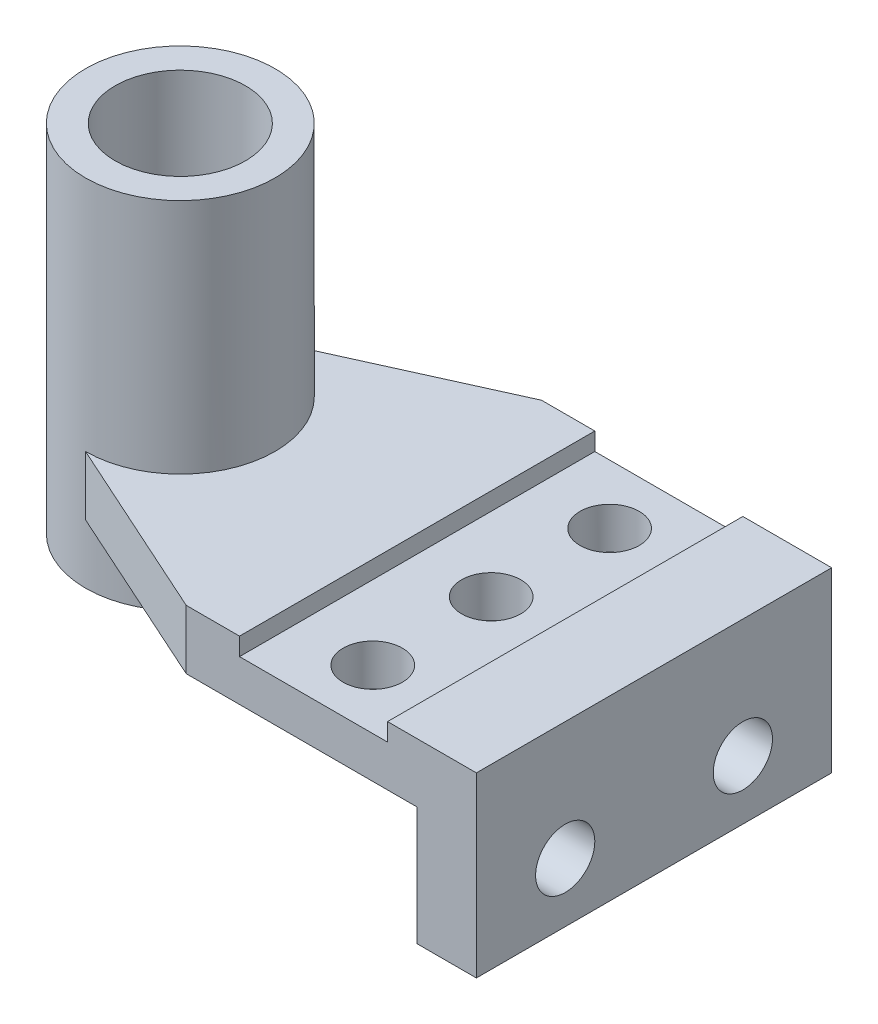
ISO-10303-21;
HEADER;
FILE_DESCRIPTION(('STEP AP214'),'2;1');
FILE_NAME('part.step','',(''),(''),'','','');
FILE_SCHEMA(('AUTOMOTIVE_DESIGN { 1 0 10303 214 1 1 1 1 }'));
ENDSEC;
DATA;
#1=APPLICATION_CONTEXT('core data for automotive mechanical design processes');
#2=APPLICATION_PROTOCOL_DEFINITION('international standard','automotive_design',2000,#1);
#3=PRODUCT_CONTEXT('',#1,'mechanical');
#4=PRODUCT('Part','Part','',(#3));
#5=PRODUCT_RELATED_PRODUCT_CATEGORY('part','',(#4));
#6=PRODUCT_DEFINITION_FORMATION('','',#4);
#7=PRODUCT_DEFINITION_CONTEXT('part definition',#1,'design');
#8=PRODUCT_DEFINITION('design','',#6,#7);
#9=PRODUCT_DEFINITION_SHAPE('','',#8);
#10=(LENGTH_UNIT() NAMED_UNIT(*) SI_UNIT(.MILLI.,.METRE.));
#11=(NAMED_UNIT(*) PLANE_ANGLE_UNIT() SI_UNIT($,.RADIAN.));
#12=(NAMED_UNIT(*) SI_UNIT($,.STERADIAN.) SOLID_ANGLE_UNIT());
#13=UNCERTAINTY_MEASURE_WITH_UNIT(LENGTH_MEASURE(1.E-05),#10,'distance_accuracy_value','');
#14=(GEOMETRIC_REPRESENTATION_CONTEXT(3) GLOBAL_UNCERTAINTY_ASSIGNED_CONTEXT((#13)) GLOBAL_UNIT_ASSIGNED_CONTEXT((#10,
#11,#12)) REPRESENTATION_CONTEXT('',''));
#15=CARTESIAN_POINT('',(0.,0.,0.));
#16=DIRECTION('',(0.,0.,1.));
#17=DIRECTION('',(1.,0.,0.));
#18=AXIS2_PLACEMENT_3D('',#15,#16,#17);
#19=CARTESIAN_POINT('',(0.,0.,30.));
#20=DIRECTION('',(0.,1.,0.));
#21=DIRECTION('',(0.,0.,1.));
#22=AXIS2_PLACEMENT_3D('',#19,#20,#21);
#23=PLANE('',#22);
#24=CARTESIAN_POINT('',(52.5,0.,20.));
#25=DIRECTION('',(0.,1.,0.));
#26=DIRECTION('',(0.,0.,1.));
#27=AXIS2_PLACEMENT_3D('',#24,#25,#26);
#28=CIRCLE('',#27,5.);
#29=CARTESIAN_POINT('',(52.5,0.,25.));
#30=VERTEX_POINT('',#29);
#31=EDGE_CURVE('E300',#30,#30,#28,.T.);
#32=ORIENTED_EDGE('',*,*,#31,.T.);
#33=EDGE_LOOP('',(#32));
#34=FACE_BOUND('',#33,.T.);
#35=CARTESIAN_POINT('',(52.5,0.,0.));
#36=DIRECTION('',(0.,1.,0.));
#37=DIRECTION('',(0.,0.,1.));
#38=AXIS2_PLACEMENT_3D('',#35,#36,#37);
#39=CIRCLE('',#38,5.);
#40=CARTESIAN_POINT('',(52.5,0.,5.));
#41=VERTEX_POINT('',#40);
#42=EDGE_CURVE('E301',#41,#41,#39,.T.);
#43=ORIENTED_EDGE('',*,*,#42,.T.);
#44=EDGE_LOOP('',(#43));
#45=FACE_BOUND('',#44,.T.);
#46=CARTESIAN_POINT('',(52.5,0.,-20.));
#47=DIRECTION('',(0.,1.,0.));
#48=DIRECTION('',(0.,0.,1.));
#49=AXIS2_PLACEMENT_3D('',#46,#47,#48);
#50=CIRCLE('',#49,5.);
#51=CARTESIAN_POINT('',(52.5,0.,-15.));
#52=VERTEX_POINT('',#51);
#53=EDGE_CURVE('E303',#52,#52,#50,.T.);
#54=ORIENTED_EDGE('',*,*,#53,.T.);
#55=EDGE_LOOP('',(#54));
#56=FACE_BOUND('',#55,.T.);
#57=DIRECTION('',(-0.911370599658675,0.,-0.411586722426498));
#58=VECTOR('',#57,1.);
#59=CARTESIAN_POINT('',(5.25151253241141,0.,18.371650821089));
#60=LINE('',#59,#58);
#61=CARTESIAN_POINT('',(31.,0.,30.));
#62=VERTEX_POINT('',#61);
#63=CARTESIAN_POINT('',(0.,0.,16.));
#64=VERTEX_POINT('',#63);
#65=EDGE_CURVE('E55',#62,#64,#60,.T.);
#66=ORIENTED_EDGE('',*,*,#65,.T.);
#67=CARTESIAN_POINT('',(0.,0.,0.));
#68=DIRECTION('',(0.,1.,0.));
#69=DIRECTION('',(0.,0.,1.));
#70=AXIS2_PLACEMENT_3D('',#67,#68,#69);
#71=CIRCLE('',#70,16.);
#72=CARTESIAN_POINT('',(0.,0.,-16.));
#73=VERTEX_POINT('',#72);
#74=EDGE_CURVE('E231',#64,#73,#71,.T.);
#75=ORIENTED_EDGE('',*,*,#74,.T.);
#76=DIRECTION('',(-0.911370599658675,0.,0.411586722426498));
#77=VECTOR('',#76,1.);
#78=CARTESIAN_POINT('',(-17.2549697493518,0.,-8.20743301642179));
#79=LINE('',#78,#77);
#80=CARTESIAN_POINT('',(31.,0.,-30.));
#81=VERTEX_POINT('',#80);
#82=EDGE_CURVE('E142',#81,#73,#79,.T.);
#83=ORIENTED_EDGE('',*,*,#82,.F.);
#84=DIRECTION('',(1.,0.,0.));
#85=VECTOR('',#84,1.);
#86=CARTESIAN_POINT('',(0.,0.,-30.));
#87=LINE('',#86,#85);
#88=CARTESIAN_POINT('',(70.,0.,-30.));
#89=VERTEX_POINT('',#88);
#90=EDGE_CURVE('E166',#81,#89,#87,.T.);
#91=ORIENTED_EDGE('',*,*,#90,.T.);
#92=DIRECTION('',(0.,0.,-1.));
#93=VECTOR('',#92,1.);
#94=CARTESIAN_POINT('',(70.,0.,30.));
#95=LINE('',#94,#93);
#96=CARTESIAN_POINT('',(70.,0.,30.));
#97=VERTEX_POINT('',#96);
#98=EDGE_CURVE('E223',#97,#89,#95,.T.);
#99=ORIENTED_EDGE('',*,*,#98,.F.);
#100=DIRECTION('',(1.,0.,0.));
#101=VECTOR('',#100,1.);
#102=CARTESIAN_POINT('',(0.,0.,30.));
#103=LINE('',#102,#101);
#104=EDGE_CURVE('E168',#62,#97,#103,.T.);
#105=ORIENTED_EDGE('',*,*,#104,.F.);
#106=EDGE_LOOP('',(#66,#75,#83,#91,#99,#105));
#107=FACE_BOUND('',#106,.T.);
#108=ADVANCED_FACE('F39',(#34,#45,#56,#107),#23,.F.);
#109=CARTESIAN_POINT('',(0.,10.,30.));
#110=DIRECTION('',(0.,-1.,0.));
#111=DIRECTION('',(0.,0.,-1.));
#112=AXIS2_PLACEMENT_3D('',#109,#110,#111);
#113=PLANE('',#112);
#114=CARTESIAN_POINT('',(0.,10.,0.));
#115=DIRECTION('',(0.,1.,0.));
#116=DIRECTION('',(0.,0.,1.));
#117=AXIS2_PLACEMENT_3D('',#114,#115,#116);
#118=CIRCLE('',#117,16.);
#119=CARTESIAN_POINT('',(0.,10.,16.));
#120=VERTEX_POINT('',#119);
#121=CARTESIAN_POINT('',(0.,10.,-16.));
#122=VERTEX_POINT('',#121);
#123=EDGE_CURVE('E130',#120,#122,#118,.T.);
#124=ORIENTED_EDGE('',*,*,#123,.F.);
#125=DIRECTION('',(-0.911370599658675,0.,-0.411586722426498));
#126=VECTOR('',#125,1.);
#127=CARTESIAN_POINT('',(-6.00172860847018,10.,13.2895419187554));
#128=LINE('',#127,#126);
#129=CARTESIAN_POINT('',(31.,10.,30.));
#130=VERTEX_POINT('',#129);
#131=EDGE_CURVE('E147',#130,#120,#128,.T.);
#132=ORIENTED_EDGE('',*,*,#131,.F.);
#133=DIRECTION('',(-1.,0.,0.));
#134=VECTOR('',#133,1.);
#135=CARTESIAN_POINT('',(0.,10.,30.));
#136=LINE('',#135,#134);
#137=CARTESIAN_POINT('',(40.,10.,30.));
#138=VERTEX_POINT('',#137);
#139=EDGE_CURVE('E188',#138,#130,#136,.T.);
#140=ORIENTED_EDGE('',*,*,#139,.F.);
#141=DIRECTION('',(0.,0.,-1.));
#142=VECTOR('',#141,1.);
#143=CARTESIAN_POINT('',(40.,10.,30.));
#144=LINE('',#143,#142);
#145=CARTESIAN_POINT('',(40.,10.,-30.));
#146=VERTEX_POINT('',#145);
#147=EDGE_CURVE('E187',#138,#146,#144,.T.);
#148=ORIENTED_EDGE('',*,*,#147,.T.);
#149=DIRECTION('',(-1.,0.,0.));
#150=VECTOR('',#149,1.);
#151=CARTESIAN_POINT('',(0.,10.,-30.));
#152=LINE('',#151,#150);
#153=CARTESIAN_POINT('',(31.,10.,-30.));
#154=VERTEX_POINT('',#153);
#155=EDGE_CURVE('E146',#146,#154,#152,.T.);
#156=ORIENTED_EDGE('',*,*,#155,.T.);
#157=DIRECTION('',(-0.911370599658675,0.,0.411586722426498));
#158=VECTOR('',#157,1.);
#159=CARTESIAN_POINT('',(-6.00172860847018,10.,-13.2895419187554));
#160=LINE('',#159,#158);
#161=EDGE_CURVE('E58',#154,#122,#160,.T.);
#162=ORIENTED_EDGE('',*,*,#161,.T.);
#163=EDGE_LOOP('',(#124,#132,#140,#148,#156,#162));
#164=FACE_BOUND('',#163,.T.);
#165=ADVANCED_FACE('F144',(#164),#113,.F.);
#166=CARTESIAN_POINT('',(0.,0.,-30.));
#167=DIRECTION('',(0.,0.,1.));
#168=DIRECTION('',(1.,0.,0.));
#169=AXIS2_PLACEMENT_3D('',#166,#167,#168);
#170=PLANE('',#169);
#171=DIRECTION('',(0.,-1.,0.));
#172=VECTOR('',#171,1.);
#173=CARTESIAN_POINT('',(31.,0.,-30.));
#174=LINE('',#173,#172);
#175=EDGE_CURVE('E46',#154,#81,#174,.T.);
#176=ORIENTED_EDGE('',*,*,#175,.F.);
#177=ORIENTED_EDGE('',*,*,#155,.F.);
#178=DIRECTION('',(0.,1.,0.));
#179=VECTOR('',#178,1.);
#180=CARTESIAN_POINT('',(40.,10.,-30.));
#181=LINE('',#180,#179);
#182=CARTESIAN_POINT('',(40.,7.,-30.));
#183=VERTEX_POINT('',#182);
#184=EDGE_CURVE('E201',#183,#146,#181,.T.);
#185=ORIENTED_EDGE('',*,*,#184,.F.);
#186=DIRECTION('',(-1.,0.,0.));
#187=VECTOR('',#186,1.);
#188=CARTESIAN_POINT('',(40.,7.,-30.));
#189=LINE('',#188,#187);
#190=CARTESIAN_POINT('',(65.,7.,-30.));
#191=VERTEX_POINT('',#190);
#192=EDGE_CURVE('E203',#191,#183,#189,.T.);
#193=ORIENTED_EDGE('',*,*,#192,.F.);
#194=DIRECTION('',(0.,-1.,0.));
#195=VECTOR('',#194,1.);
#196=CARTESIAN_POINT('',(65.,7.,-30.));
#197=LINE('',#196,#195);
#198=CARTESIAN_POINT('',(65.,10.,-30.));
#199=VERTEX_POINT('',#198);
#200=EDGE_CURVE('E200',#199,#191,#197,.T.);
#201=ORIENTED_EDGE('',*,*,#200,.F.);
#202=DIRECTION('',(-1.,0.,0.));
#203=VECTOR('',#202,1.);
#204=CARTESIAN_POINT('',(65.,10.,-30.));
#205=LINE('',#204,#203);
#206=CARTESIAN_POINT('',(80.,10.,-30.));
#207=VERTEX_POINT('',#206);
#208=EDGE_CURVE('E197',#207,#199,#205,.T.);
#209=ORIENTED_EDGE('',*,*,#208,.F.);
#210=DIRECTION('',(0.,1.,0.));
#211=VECTOR('',#210,1.);
#212=CARTESIAN_POINT('',(80.,-20.,-30.));
#213=LINE('',#212,#211);
#214=CARTESIAN_POINT('',(80.,-20.,-30.));
#215=VERTEX_POINT('',#214);
#216=EDGE_CURVE('E194',#215,#207,#213,.T.);
#217=ORIENTED_EDGE('',*,*,#216,.F.);
#218=DIRECTION('',(1.,0.,0.));
#219=VECTOR('',#218,1.);
#220=CARTESIAN_POINT('',(70.,-20.,-30.));
#221=LINE('',#220,#219);
#222=CARTESIAN_POINT('',(70.,-20.,-30.));
#223=VERTEX_POINT('',#222);
#224=EDGE_CURVE('E192',#223,#215,#221,.T.);
#225=ORIENTED_EDGE('',*,*,#224,.F.);
#226=DIRECTION('',(0.,-1.,0.));
#227=VECTOR('',#226,1.);
#228=CARTESIAN_POINT('',(70.,0.,-30.));
#229=LINE('',#228,#227);
#230=EDGE_CURVE('E191',#89,#223,#229,.T.);
#231=ORIENTED_EDGE('',*,*,#230,.F.);
#232=ORIENTED_EDGE('',*,*,#90,.F.);
#233=EDGE_LOOP('',(#176,#177,#185,#193,#201,#209,#217,#225,#231,#232));
#234=FACE_BOUND('',#233,.T.);
#235=ADVANCED_FACE('F232',(#234),#170,.F.);
#236=CARTESIAN_POINT('',(70.,0.,30.));
#237=DIRECTION('',(1.,0.,0.));
#238=DIRECTION('',(0.,0.,-1.));
#239=AXIS2_PLACEMENT_3D('',#236,#237,#238);
#240=PLANE('',#239);
#241=CARTESIAN_POINT('',(70.,-10.,15.));
#242=DIRECTION('',(1.,0.,0.));
#243=DIRECTION('',(0.,0.,-1.));
#244=AXIS2_PLACEMENT_3D('',#241,#242,#243);
#245=CIRCLE('',#244,5.);
#246=CARTESIAN_POINT('',(70.,-10.,10.));
#247=VERTEX_POINT('',#246);
#248=EDGE_CURVE('E167',#247,#247,#245,.T.);
#249=ORIENTED_EDGE('',*,*,#248,.T.);
#250=EDGE_LOOP('',(#249));
#251=FACE_BOUND('',#250,.T.);
#252=CARTESIAN_POINT('',(70.,-10.,-15.));
#253=DIRECTION('',(1.,0.,0.));
#254=DIRECTION('',(0.,0.,-1.));
#255=AXIS2_PLACEMENT_3D('',#252,#253,#254);
#256=CIRCLE('',#255,5.);
#257=CARTESIAN_POINT('',(70.,-10.,-20.));
#258=VERTEX_POINT('',#257);
#259=EDGE_CURVE('E161',#258,#258,#256,.T.);
#260=ORIENTED_EDGE('',*,*,#259,.T.);
#261=EDGE_LOOP('',(#260));
#262=FACE_BOUND('',#261,.T.);
#263=ORIENTED_EDGE('',*,*,#230,.T.);
#264=DIRECTION('',(0.,0.,-1.));
#265=VECTOR('',#264,1.);
#266=CARTESIAN_POINT('',(70.,-20.,30.));
#267=LINE('',#266,#265);
#268=CARTESIAN_POINT('',(70.,-20.,30.));
#269=VERTEX_POINT('',#268);
#270=EDGE_CURVE('E225',#269,#223,#267,.T.);
#271=ORIENTED_EDGE('',*,*,#270,.F.);
#272=DIRECTION('',(0.,-1.,0.));
#273=VECTOR('',#272,1.);
#274=CARTESIAN_POINT('',(70.,0.,30.));
#275=LINE('',#274,#273);
#276=EDGE_CURVE('E175',#97,#269,#275,.T.);
#277=ORIENTED_EDGE('',*,*,#276,.F.);
#278=ORIENTED_EDGE('',*,*,#98,.T.);
#279=EDGE_LOOP('',(#263,#271,#277,#278));
#280=FACE_BOUND('',#279,.T.);
#281=ADVANCED_FACE('F236',(#251,#262,#280),#240,.F.);
#282=CARTESIAN_POINT('',(70.,-20.,30.));
#283=DIRECTION('',(0.,1.,0.));
#284=DIRECTION('',(0.,0.,1.));
#285=AXIS2_PLACEMENT_3D('',#282,#283,#284);
#286=PLANE('',#285);
#287=ORIENTED_EDGE('',*,*,#224,.T.);
#288=DIRECTION('',(0.,0.,-1.));
#289=VECTOR('',#288,1.);
#290=CARTESIAN_POINT('',(80.,-20.,30.));
#291=LINE('',#290,#289);
#292=CARTESIAN_POINT('',(80.,-20.,30.));
#293=VERTEX_POINT('',#292);
#294=EDGE_CURVE('E218',#293,#215,#291,.T.);
#295=ORIENTED_EDGE('',*,*,#294,.F.);
#296=DIRECTION('',(1.,0.,0.));
#297=VECTOR('',#296,1.);
#298=CARTESIAN_POINT('',(70.,-20.,30.));
#299=LINE('',#298,#297);
#300=EDGE_CURVE('E172',#269,#293,#299,.T.);
#301=ORIENTED_EDGE('',*,*,#300,.F.);
#302=ORIENTED_EDGE('',*,*,#270,.T.);
#303=EDGE_LOOP('',(#287,#295,#301,#302));
#304=FACE_BOUND('',#303,.T.);
#305=ADVANCED_FACE('F245',(#304),#286,.F.);
#306=CARTESIAN_POINT('',(80.,-20.,30.));
#307=DIRECTION('',(-1.,0.,0.));
#308=DIRECTION('',(0.,0.,1.));
#309=AXIS2_PLACEMENT_3D('',#306,#307,#308);
#310=PLANE('',#309);
#311=CARTESIAN_POINT('',(80.,-10.,15.));
#312=DIRECTION('',(1.,0.,0.));
#313=DIRECTION('',(0.,0.,-1.));
#314=AXIS2_PLACEMENT_3D('',#311,#312,#313);
#315=CIRCLE('',#314,5.);
#316=CARTESIAN_POINT('',(80.,-10.,10.));
#317=VERTEX_POINT('',#316);
#318=EDGE_CURVE('E158',#317,#317,#315,.T.);
#319=ORIENTED_EDGE('',*,*,#318,.F.);
#320=EDGE_LOOP('',(#319));
#321=FACE_BOUND('',#320,.T.);
#322=CARTESIAN_POINT('',(80.,-10.,-15.));
#323=DIRECTION('',(1.,0.,0.));
#324=DIRECTION('',(0.,0.,-1.));
#325=AXIS2_PLACEMENT_3D('',#322,#323,#324);
#326=CIRCLE('',#325,5.);
#327=CARTESIAN_POINT('',(80.,-10.,-20.));
#328=VERTEX_POINT('',#327);
#329=EDGE_CURVE('E160',#328,#328,#326,.T.);
#330=ORIENTED_EDGE('',*,*,#329,.F.);
#331=EDGE_LOOP('',(#330));
#332=FACE_BOUND('',#331,.T.);
#333=ORIENTED_EDGE('',*,*,#216,.T.);
#334=DIRECTION('',(0.,0.,-1.));
#335=VECTOR('',#334,1.);
#336=CARTESIAN_POINT('',(80.,10.,30.));
#337=LINE('',#336,#335);
#338=CARTESIAN_POINT('',(80.,10.,30.));
#339=VERTEX_POINT('',#338);
#340=EDGE_CURVE('E216',#339,#207,#337,.T.);
#341=ORIENTED_EDGE('',*,*,#340,.F.);
#342=DIRECTION('',(0.,1.,0.));
#343=VECTOR('',#342,1.);
#344=CARTESIAN_POINT('',(80.,-20.,30.));
#345=LINE('',#344,#343);
#346=EDGE_CURVE('E176',#293,#339,#345,.T.);
#347=ORIENTED_EDGE('',*,*,#346,.F.);
#348=ORIENTED_EDGE('',*,*,#294,.T.);
#349=EDGE_LOOP('',(#333,#341,#347,#348));
#350=FACE_BOUND('',#349,.T.);
#351=ADVANCED_FACE('F275',(#321,#332,#350),#310,.F.);
#352=CARTESIAN_POINT('',(65.,10.,30.));
#353=DIRECTION('',(0.,-1.,0.));
#354=DIRECTION('',(0.,0.,-1.));
#355=AXIS2_PLACEMENT_3D('',#352,#353,#354);
#356=PLANE('',#355);
#357=ORIENTED_EDGE('',*,*,#208,.T.);
#358=DIRECTION('',(0.,0.,-1.));
#359=VECTOR('',#358,1.);
#360=CARTESIAN_POINT('',(65.,10.,30.));
#361=LINE('',#360,#359);
#362=CARTESIAN_POINT('',(65.,10.,30.));
#363=VERTEX_POINT('',#362);
#364=EDGE_CURVE('E213',#363,#199,#361,.T.);
#365=ORIENTED_EDGE('',*,*,#364,.F.);
#366=DIRECTION('',(-1.,0.,0.));
#367=VECTOR('',#366,1.);
#368=CARTESIAN_POINT('',(65.,10.,30.));
#369=LINE('',#368,#367);
#370=EDGE_CURVE('E177',#339,#363,#369,.T.);
#371=ORIENTED_EDGE('',*,*,#370,.F.);
#372=ORIENTED_EDGE('',*,*,#340,.T.);
#373=EDGE_LOOP('',(#357,#365,#371,#372));
#374=FACE_BOUND('',#373,.T.);
#375=ADVANCED_FACE('F267',(#374),#356,.F.);
#376=CARTESIAN_POINT('',(65.,7.,30.));
#377=DIRECTION('',(1.,0.,0.));
#378=DIRECTION('',(0.,0.,-1.));
#379=AXIS2_PLACEMENT_3D('',#376,#377,#378);
#380=PLANE('',#379);
#381=ORIENTED_EDGE('',*,*,#200,.T.);
#382=DIRECTION('',(0.,0.,-1.));
#383=VECTOR('',#382,1.);
#384=CARTESIAN_POINT('',(65.,7.,30.));
#385=LINE('',#384,#383);
#386=CARTESIAN_POINT('',(65.,7.,30.));
#387=VERTEX_POINT('',#386);
#388=EDGE_CURVE('E209',#387,#191,#385,.T.);
#389=ORIENTED_EDGE('',*,*,#388,.F.);
#390=DIRECTION('',(0.,-1.,0.));
#391=VECTOR('',#390,1.);
#392=CARTESIAN_POINT('',(65.,7.,30.));
#393=LINE('',#392,#391);
#394=EDGE_CURVE('E179',#363,#387,#393,.T.);
#395=ORIENTED_EDGE('',*,*,#394,.F.);
#396=ORIENTED_EDGE('',*,*,#364,.T.);
#397=EDGE_LOOP('',(#381,#389,#395,#396));
#398=FACE_BOUND('',#397,.T.);
#399=ADVANCED_FACE('F264',(#398),#380,.F.);
#400=CARTESIAN_POINT('',(40.,7.,30.));
#401=DIRECTION('',(0.,-1.,0.));
#402=DIRECTION('',(0.,0.,-1.));
#403=AXIS2_PLACEMENT_3D('',#400,#401,#402);
#404=PLANE('',#403);
#405=CARTESIAN_POINT('',(52.5,7.,20.));
#406=DIRECTION('',(0.,1.,0.));
#407=DIRECTION('',(0.,0.,1.));
#408=AXIS2_PLACEMENT_3D('',#405,#406,#407);
#409=CIRCLE('',#408,5.);
#410=CARTESIAN_POINT('',(52.5,7.,25.));
#411=VERTEX_POINT('',#410);
#412=EDGE_CURVE('E308',#411,#411,#409,.T.);
#413=ORIENTED_EDGE('',*,*,#412,.F.);
#414=EDGE_LOOP('',(#413));
#415=FACE_BOUND('',#414,.T.);
#416=CARTESIAN_POINT('',(52.5,7.,0.));
#417=DIRECTION('',(0.,1.,0.));
#418=DIRECTION('',(0.,0.,1.));
#419=AXIS2_PLACEMENT_3D('',#416,#417,#418);
#420=CIRCLE('',#419,5.);
#421=CARTESIAN_POINT('',(52.5,7.,5.));
#422=VERTEX_POINT('',#421);
#423=EDGE_CURVE('E309',#422,#422,#420,.T.);
#424=ORIENTED_EDGE('',*,*,#423,.F.);
#425=EDGE_LOOP('',(#424));
#426=FACE_BOUND('',#425,.T.);
#427=CARTESIAN_POINT('',(52.5,7.,-20.));
#428=DIRECTION('',(0.,1.,0.));
#429=DIRECTION('',(0.,0.,-1.));
#430=AXIS2_PLACEMENT_3D('',#427,#428,#429);
#431=CIRCLE('',#430,5.);
#432=CARTESIAN_POINT('',(52.5,7.,-25.));
#433=VERTEX_POINT('',#432);
#434=EDGE_CURVE('E311',#433,#433,#431,.T.);
#435=ORIENTED_EDGE('',*,*,#434,.F.);
#436=EDGE_LOOP('',(#435));
#437=FACE_BOUND('',#436,.T.);
#438=ORIENTED_EDGE('',*,*,#192,.T.);
#439=DIRECTION('',(0.,0.,-1.));
#440=VECTOR('',#439,1.);
#441=CARTESIAN_POINT('',(40.,7.,30.));
#442=LINE('',#441,#440);
#443=CARTESIAN_POINT('',(40.,7.,30.));
#444=VERTEX_POINT('',#443);
#445=EDGE_CURVE('E210',#444,#183,#442,.T.);
#446=ORIENTED_EDGE('',*,*,#445,.F.);
#447=DIRECTION('',(-1.,0.,0.));
#448=VECTOR('',#447,1.);
#449=CARTESIAN_POINT('',(40.,7.,30.));
#450=LINE('',#449,#448);
#451=EDGE_CURVE('E185',#387,#444,#450,.T.);
#452=ORIENTED_EDGE('',*,*,#451,.F.);
#453=ORIENTED_EDGE('',*,*,#388,.T.);
#454=EDGE_LOOP('',(#438,#446,#452,#453));
#455=FACE_BOUND('',#454,.T.);
#456=ADVANCED_FACE('F261',(#415,#426,#437,#455),#404,.F.);
#457=CARTESIAN_POINT('',(40.,10.,30.));
#458=DIRECTION('',(-1.,0.,0.));
#459=DIRECTION('',(0.,0.,1.));
#460=AXIS2_PLACEMENT_3D('',#457,#458,#459);
#461=PLANE('',#460);
#462=ORIENTED_EDGE('',*,*,#184,.T.);
#463=ORIENTED_EDGE('',*,*,#147,.F.);
#464=DIRECTION('',(0.,1.,0.));
#465=VECTOR('',#464,1.);
#466=CARTESIAN_POINT('',(40.,10.,30.));
#467=LINE('',#466,#465);
#468=EDGE_CURVE('E184',#444,#138,#467,.T.);
#469=ORIENTED_EDGE('',*,*,#468,.F.);
#470=ORIENTED_EDGE('',*,*,#445,.T.);
#471=EDGE_LOOP('',(#462,#463,#469,#470));
#472=FACE_BOUND('',#471,.T.);
#473=ADVANCED_FACE('F260',(#472),#461,.F.);
#474=CARTESIAN_POINT('',(0.,0.,30.));
#475=DIRECTION('',(0.,0.,1.));
#476=DIRECTION('',(1.,0.,0.));
#477=AXIS2_PLACEMENT_3D('',#474,#475,#476);
#478=PLANE('',#477);
#479=DIRECTION('',(0.,1.,0.));
#480=VECTOR('',#479,1.);
#481=CARTESIAN_POINT('',(31.,0.,30.));
#482=LINE('',#481,#480);
#483=EDGE_CURVE('E11',#62,#130,#482,.T.);
#484=ORIENTED_EDGE('',*,*,#483,.F.);
#485=ORIENTED_EDGE('',*,*,#104,.T.);
#486=ORIENTED_EDGE('',*,*,#276,.T.);
#487=ORIENTED_EDGE('',*,*,#300,.T.);
#488=ORIENTED_EDGE('',*,*,#346,.T.);
#489=ORIENTED_EDGE('',*,*,#370,.T.);
#490=ORIENTED_EDGE('',*,*,#394,.T.);
#491=ORIENTED_EDGE('',*,*,#451,.T.);
#492=ORIENTED_EDGE('',*,*,#468,.T.);
#493=ORIENTED_EDGE('',*,*,#139,.T.);
#494=EDGE_LOOP('',(#484,#485,#486,#487,#488,#489,#490,#491,#492,#493));
#495=FACE_BOUND('',#494,.T.);
#496=ADVANCED_FACE('F246',(#495),#478,.T.);
#497=CARTESIAN_POINT('',(65.,-10.,-15.));
#498=DIRECTION('',(1.,0.,0.));
#499=DIRECTION('',(0.,0.,-1.));
#500=AXIS2_PLACEMENT_3D('',#497,#498,#499);
#501=CYLINDRICAL_SURFACE('',#500,5.);
#502=ORIENTED_EDGE('',*,*,#329,.T.);
#503=EDGE_LOOP('',(#502));
#504=FACE_BOUND('',#503,.T.);
#505=ORIENTED_EDGE('',*,*,#259,.F.);
#506=EDGE_LOOP('',(#505));
#507=FACE_BOUND('',#506,.T.);
#508=ADVANCED_FACE('F348',(#504,#507),#501,.F.);
#509=CARTESIAN_POINT('',(65.,-10.,15.));
#510=DIRECTION('',(1.,0.,0.));
#511=DIRECTION('',(0.,0.,-1.));
#512=AXIS2_PLACEMENT_3D('',#509,#510,#511);
#513=CYLINDRICAL_SURFACE('',#512,5.);
#514=ORIENTED_EDGE('',*,*,#318,.T.);
#515=EDGE_LOOP('',(#514));
#516=FACE_BOUND('',#515,.T.);
#517=ORIENTED_EDGE('',*,*,#248,.F.);
#518=EDGE_LOOP('',(#517));
#519=FACE_BOUND('',#518,.T.);
#520=ADVANCED_FACE('F347',(#516,#519),#513,.F.);
#521=CARTESIAN_POINT('',(-6.00172860847018,-5.,-13.2895419187554));
#522=DIRECTION('',(-0.411586722426498,0.,-0.911370599658675));
#523=DIRECTION('',(-0.911370599658675,0.,0.411586722426498));
#524=AXIS2_PLACEMENT_3D('',#521,#522,#523);
#525=PLANE('',#524);
#526=ORIENTED_EDGE('',*,*,#82,.T.);
#527=DIRECTION('',(0.,1.,0.));
#528=VECTOR('',#527,1.);
#529=CARTESIAN_POINT('',(0.,-5.,-16.));
#530=LINE('',#529,#528);
#531=EDGE_CURVE('E128',#73,#122,#530,.T.);
#532=ORIENTED_EDGE('',*,*,#531,.T.);
#533=ORIENTED_EDGE('',*,*,#161,.F.);
#534=ORIENTED_EDGE('',*,*,#175,.T.);
#535=EDGE_LOOP('',(#526,#532,#533,#534));
#536=FACE_BOUND('',#535,.T.);
#537=ADVANCED_FACE('F139',(#536),#525,.T.);
#538=CARTESIAN_POINT('',(-6.00172860847018,-5.,13.2895419187554));
#539=DIRECTION('',(0.411586722426498,0.,-0.911370599658675));
#540=DIRECTION('',(-0.911370599658675,0.,-0.411586722426498));
#541=AXIS2_PLACEMENT_3D('',#538,#539,#540);
#542=PLANE('',#541);
#543=ORIENTED_EDGE('',*,*,#483,.T.);
#544=ORIENTED_EDGE('',*,*,#131,.T.);
#545=DIRECTION('',(0.,1.,0.));
#546=VECTOR('',#545,1.);
#547=CARTESIAN_POINT('',(0.,-5.,16.));
#548=LINE('',#547,#546);
#549=EDGE_CURVE('E135',#64,#120,#548,.T.);
#550=ORIENTED_EDGE('',*,*,#549,.F.);
#551=ORIENTED_EDGE('',*,*,#65,.F.);
#552=EDGE_LOOP('',(#543,#544,#550,#551));
#553=FACE_BOUND('',#552,.T.);
#554=ADVANCED_FACE('F249',(#553),#542,.F.);
#555=CARTESIAN_POINT('',(0.,50.,0.));
#556=DIRECTION('',(0.,1.,0.));
#557=DIRECTION('',(0.,0.,1.));
#558=AXIS2_PLACEMENT_3D('',#555,#556,#557);
#559=PLANE('',#558);
#560=CARTESIAN_POINT('',(0.,50.,0.));
#561=DIRECTION('',(0.,1.,0.));
#562=DIRECTION('',(0.,0.,1.));
#563=AXIS2_PLACEMENT_3D('',#560,#561,#562);
#564=CIRCLE('',#563,16.);
#565=CARTESIAN_POINT('',(0.,50.,16.));
#566=VERTEX_POINT('',#565);
#567=EDGE_CURVE('E136',#566,#566,#564,.T.);
#568=ORIENTED_EDGE('',*,*,#567,.T.);
#569=EDGE_LOOP('',(#568));
#570=FACE_BOUND('',#569,.T.);
#571=CARTESIAN_POINT('',(0.,50.,0.));
#572=DIRECTION('',(0.,1.,0.));
#573=DIRECTION('',(0.,0.,1.));
#574=AXIS2_PLACEMENT_3D('',#571,#572,#573);
#575=CIRCLE('',#574,11.);
#576=CARTESIAN_POINT('',(0.,50.,11.));
#577=VERTEX_POINT('',#576);
#578=EDGE_CURVE('E140',#577,#577,#575,.T.);
#579=ORIENTED_EDGE('',*,*,#578,.F.);
#580=EDGE_LOOP('',(#579));
#581=FACE_BOUND('',#580,.T.);
#582=ADVANCED_FACE('F327',(#570,#581),#559,.T.);
#583=CARTESIAN_POINT('',(0.,50.,0.));
#584=DIRECTION('',(0.,-1.,0.));
#585=DIRECTION('',(0.,0.,-1.));
#586=AXIS2_PLACEMENT_3D('',#583,#584,#585);
#587=CYLINDRICAL_SURFACE('',#586,16.);
#588=ORIENTED_EDGE('',*,*,#567,.F.);
#589=EDGE_LOOP('',(#588));
#590=FACE_BOUND('',#589,.T.);
#591=ORIENTED_EDGE('',*,*,#123,.T.);
#592=ORIENTED_EDGE('',*,*,#531,.F.);
#593=ORIENTED_EDGE('',*,*,#74,.F.);
#594=ORIENTED_EDGE('',*,*,#549,.T.);
#595=EDGE_LOOP('',(#591,#592,#593,#594));
#596=FACE_BOUND('',#595,.T.);
#597=CARTESIAN_POINT('',(0.,-10.,0.));
#598=DIRECTION('',(0.,1.,0.));
#599=DIRECTION('',(0.,0.,1.));
#600=AXIS2_PLACEMENT_3D('',#597,#598,#599);
#601=CIRCLE('',#600,16.);
#602=CARTESIAN_POINT('',(0.,-10.,16.));
#603=VERTEX_POINT('',#602);
#604=EDGE_CURVE('E319',#603,#603,#601,.T.);
#605=ORIENTED_EDGE('',*,*,#604,.T.);
#606=EDGE_LOOP('',(#605));
#607=FACE_BOUND('',#606,.T.);
#608=ADVANCED_FACE('F126',(#590,#596,#607),#587,.T.);
#609=CARTESIAN_POINT('',(0.,50.,0.));
#610=DIRECTION('',(0.,-1.,0.));
#611=DIRECTION('',(0.,0.,-1.));
#612=AXIS2_PLACEMENT_3D('',#609,#610,#611);
#613=CYLINDRICAL_SURFACE('',#612,11.);
#614=ORIENTED_EDGE('',*,*,#578,.T.);
#615=EDGE_LOOP('',(#614));
#616=FACE_BOUND('',#615,.T.);
#617=CARTESIAN_POINT('',(0.,-10.,0.));
#618=DIRECTION('',(0.,1.,0.));
#619=DIRECTION('',(0.,0.,1.));
#620=AXIS2_PLACEMENT_3D('',#617,#618,#619);
#621=CIRCLE('',#620,11.);
#622=CARTESIAN_POINT('',(0.,-10.,11.));
#623=VERTEX_POINT('',#622);
#624=EDGE_CURVE('E320',#623,#623,#621,.T.);
#625=ORIENTED_EDGE('',*,*,#624,.F.);
#626=EDGE_LOOP('',(#625));
#627=FACE_BOUND('',#626,.T.);
#628=ADVANCED_FACE('F335',(#616,#627),#613,.F.);
#629=CARTESIAN_POINT('',(0.,-10.,0.));
#630=DIRECTION('',(0.,1.,0.));
#631=DIRECTION('',(0.,0.,1.));
#632=AXIS2_PLACEMENT_3D('',#629,#630,#631);
#633=PLANE('',#632);
#634=ORIENTED_EDGE('',*,*,#624,.T.);
#635=EDGE_LOOP('',(#634));
#636=FACE_BOUND('',#635,.T.);
#637=ORIENTED_EDGE('',*,*,#604,.F.);
#638=EDGE_LOOP('',(#637));
#639=FACE_BOUND('',#638,.T.);
#640=ADVANCED_FACE('F336',(#636,#639),#633,.F.);
#641=CARTESIAN_POINT('',(52.5,-13.,-20.));
#642=DIRECTION('',(0.,1.,0.));
#643=DIRECTION('',(0.,0.,1.));
#644=AXIS2_PLACEMENT_3D('',#641,#642,#643);
#645=CYLINDRICAL_SURFACE('',#644,5.);
#646=ORIENTED_EDGE('',*,*,#434,.T.);
#647=EDGE_LOOP('',(#646));
#648=FACE_BOUND('',#647,.T.);
#649=ORIENTED_EDGE('',*,*,#53,.F.);
#650=EDGE_LOOP('',(#649));
#651=FACE_BOUND('',#650,.T.);
#652=ADVANCED_FACE('F462',(#648,#651),#645,.F.);
#653=CARTESIAN_POINT('',(52.5,-13.,0.));
#654=DIRECTION('',(0.,1.,0.));
#655=DIRECTION('',(0.,0.,1.));
#656=AXIS2_PLACEMENT_3D('',#653,#654,#655);
#657=CYLINDRICAL_SURFACE('',#656,5.);
#658=ORIENTED_EDGE('',*,*,#423,.T.);
#659=EDGE_LOOP('',(#658));
#660=FACE_BOUND('',#659,.T.);
#661=ORIENTED_EDGE('',*,*,#42,.F.);
#662=EDGE_LOOP('',(#661));
#663=FACE_BOUND('',#662,.T.);
#664=ADVANCED_FACE('F475',(#660,#663),#657,.F.);
#665=CARTESIAN_POINT('',(52.5,-13.,20.));
#666=DIRECTION('',(0.,1.,0.));
#667=DIRECTION('',(0.,0.,1.));
#668=AXIS2_PLACEMENT_3D('',#665,#666,#667);
#669=CYLINDRICAL_SURFACE('',#668,5.);
#670=ORIENTED_EDGE('',*,*,#412,.T.);
#671=EDGE_LOOP('',(#670));
#672=FACE_BOUND('',#671,.T.);
#673=ORIENTED_EDGE('',*,*,#31,.F.);
#674=EDGE_LOOP('',(#673));
#675=FACE_BOUND('',#674,.T.);
#676=ADVANCED_FACE('F483',(#672,#675),#669,.F.);
#677=CLOSED_SHELL('',(#108,#165,#235,#281,#305,#351,#375,#399,#456,#473,#496,#508,#520,#537,
#554,#582,#608,#628,#640,#652,#664,#676));
#678=MANIFOLD_SOLID_BREP('B2',#677);
#679=ADVANCED_BREP_SHAPE_REPRESENTATION('',(#18,#678),#14);
#680=SHAPE_DEFINITION_REPRESENTATION(#9,#679);
ENDSEC;
END-ISO-10303-21;
